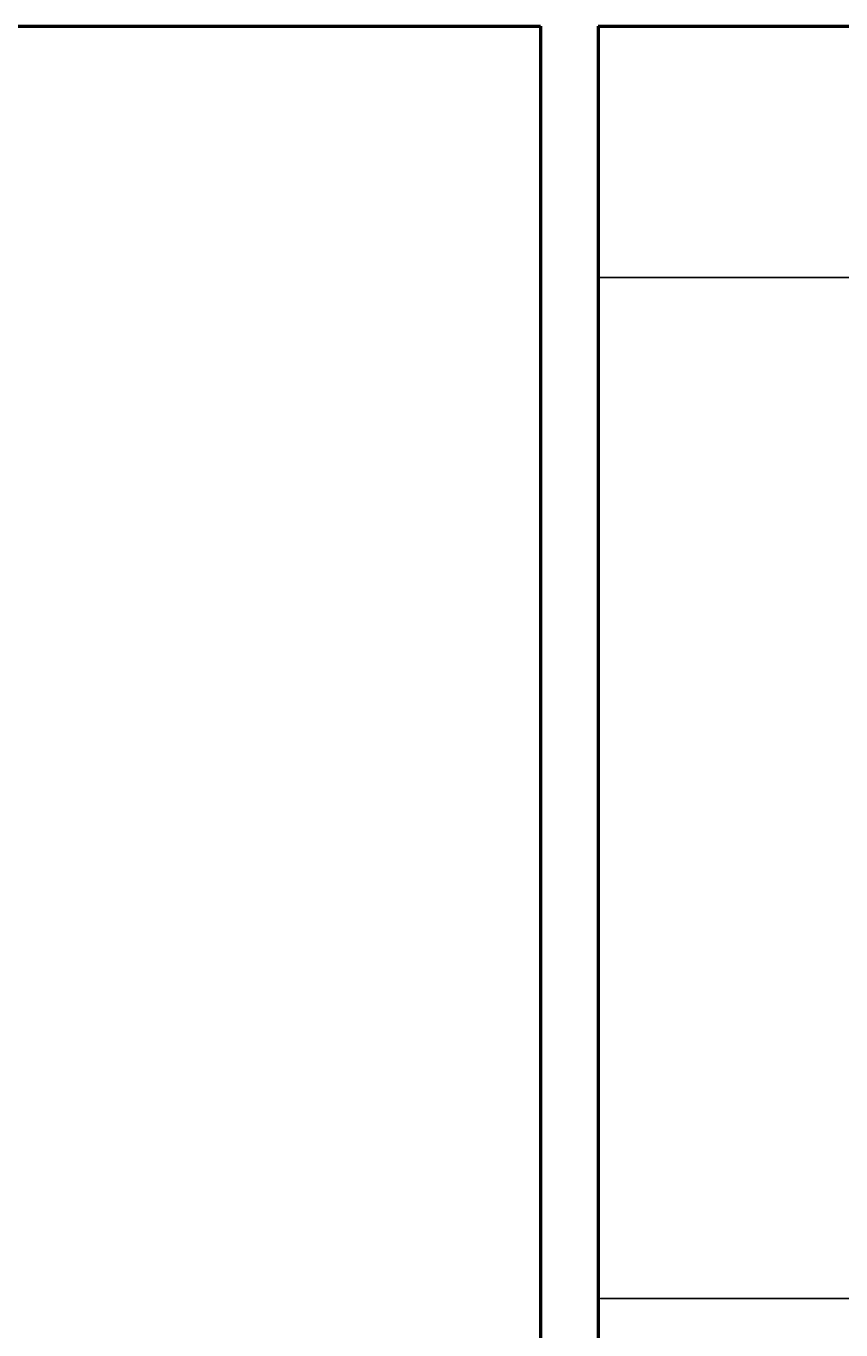
# Model space of a CAD drawing. Units: inches. Extents: x -173 to 545, y -746 to 104.
# Tile 24 of 32: x 125 to 189, y -94 to 8. Entities that reach past the tile are written whole.
import ezdxf

# ---------------------------------------------------------------- set-up
doc = ezdxf.new("R2010")
doc.units = ezdxf.units.IN
doc.header["$MEASUREMENT"] = 0
for name, color, linetype, lineweight in [('A-ANNO-DIMS', 2, 'Continuous', 18), ('A-FLOR-CASE', 9, 'Continuous', 25), ('A-WALL', 7, 'Continuous', 50)]:
    doc.layers.add(name, color=color, linetype=linetype, lineweight=lineweight)
doc.styles.get("Standard").update_dxf_attribs({"font": 'arial.ttf'})
doc.dimstyles.get("Standard").update_dxf_attribs({"dimtxt": 0.18, "dimasz": 0.18, "dimexe": 0.18, "dimexo": 0.0625, "dimgap": 0.09, "dimtad": 0, "dimtih": 1, "dimtoh": 1, "dimdec": 0, "dimzin": 0, "dimdsep": 46, "dimlunit": 3, "dimtxsty": 'Standard', "dimcen": 0.09, "dimadec": 0, "dimazin": 0, "dimtfac": 1, "dimtdec": 0, "dimtofl": 0, "dimtmove": 0, "dimatfit": 3, "dimfxl": 1, "dimtolj": 1, "dimtzin": 0, "dimarcsym": 0})

# ---------------------------------------------------------------- blocks, each defined once
blk = doc.blocks.new('COUNTER-L-RETURN')
for p, q in [((66, 69.36), (0, 69.36)), ((66, 0), (66, 69.36))]:
    blk.add_line(p, q)
blk = doc.blocks.new('*D77')
at = {"layer": 'A-ANNO-DIMS', "color": 0, "lineweight": -2, "transparency": 16777216}
for p, q in [((169.8, -81.42), (169.8, -91.95)), ((235.8, -81.42), (235.8, -91.95)), ((169.98, -91.77), (202.16, -91.77)), ((235.62, -91.77), (203.44, -91.77))]:
    blk.add_line(p, q, dxfattribs=at)
at = {"layer": 'A-ANNO-DIMS', "color": 0, "transparency": 16777216}
for points in [[(169.98, -91.74), (169.98, -91.8), (169.8, -91.77)], [(235.62, -91.74), (235.62, -91.8), (235.8, -91.77)]]:
    blk.add_solid(points, dxfattribs=at)
at = {"layer": 'Defpoints', "color": 0, "transparency": 16777216}
for p in [(169.8, -81.36), (235.8, -81.36), (235.8, -91.77)]:
    blk.add_point(p, dxfattribs=at)
at = {"layer": 'A-ANNO-DIMS', "color": 0, "transparency": 16777216, "insert": (202.8, -91.77), "char_height": 0.18, "attachment_point": 5}
blk.add_mtext('\\A1;5\'-6" TYP.', dxfattribs=at)

msp = doc.modelspace()

# ---------------------------------------------------------------- linework, layer by layer
at = {"layer": 'A-WALL'}
for p, q in [((33.3, 7.64), (165.3, 7.64)), ((165.3, 7.64), (165.3, -128.86)), ((169.8, 7.64), (169.8, -128.86)), ((169.8, 7.64), (260.8, 7.64))]:
    msp.add_line(p, q, dxfattribs=at)

# ---------------------------------------------------------------- block references
at = {"layer": 'A-FLOR-CASE'}
msp.add_blockref('COUNTER-L-RETURN', (169.8, -81.36), dxfattribs=at)

# ---------------------------------------------------------------- dimensions: what is measured, and where the dimension line sits
at = {"layer": 'A-ANNO-DIMS'}
dim = msp.add_linear_dim(base=(235.8, -91.77), p1=(169.8, -81.36), p2=(235.8, -81.36), text='<> TYP.', dimstyle='Standard', override={"dimdec": 1, "dimlfac": 1, "dimrnd": 0, "dimzin": 1, "dimdsep": 46, "dimlunit": 4, "dimfrac": 2}, dxfattribs=at)
dim.commit()
dim.dimension.update_dxf_attribs({"geometry": '*D77', "text_midpoint": (202.8, -91.77)})

doc.saveas('drawing.dxf')
